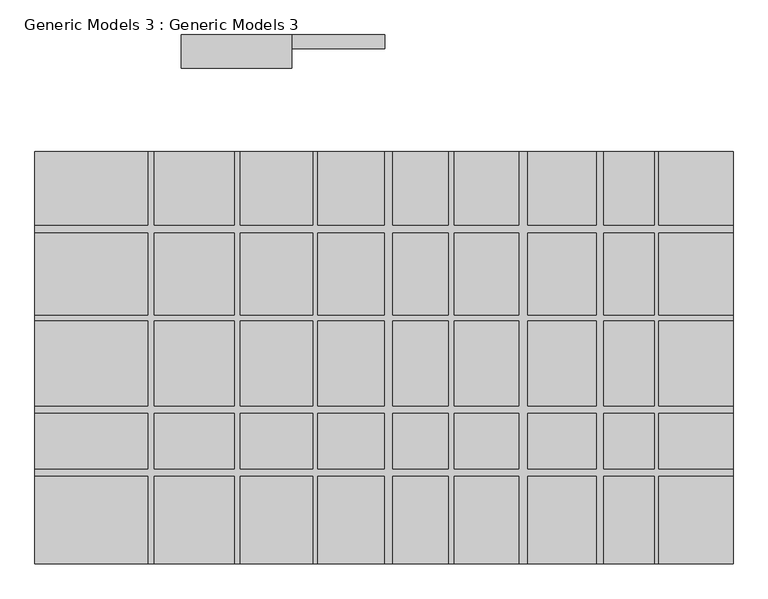
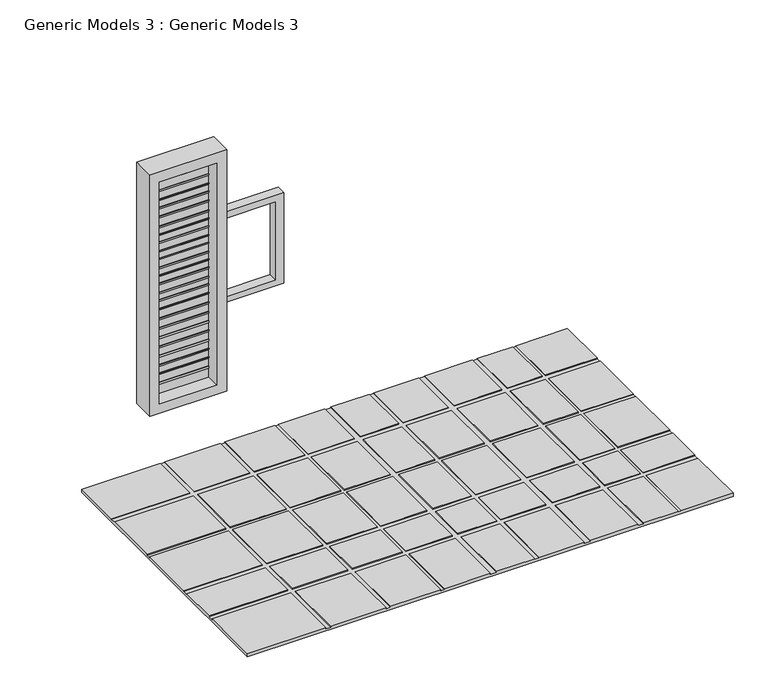
"""IFC4 building model written with IfcOpenShell, lengths in millimetres: proxy geometry, Generic Models 3 : Generic Models 3."""

from ifc_helpers import new_model, si_unit, frame, origin, place, context, project, spatial, polyline, outline, extrude, faceted_brep, source, transform, mapped, element, save


def generic_models_3_generic_models_3_2fa08359(model_context):
    return source(origin(), model_context, "Body", "SolidModel", [
        faceted_brep([(-20282.6509421, -24714.0121703, -199.9886332), (-20282.6509421, -24714.0121703, -304.8), (-4816.0838989, -24714.0121703, -304.8), (-4816.0838989, -24714.0121703, -199.9886332), (-6459.456614, -24714.0121703, -199.9886332), (-6459.456614, -24714.0121703, -225.3886332), (-6558.4876686, -24714.0121703, -225.3886332), (-6558.4876686, -24714.0121703, -199.9886332), (-7682.5837988, -24714.0121703, -199.9886332), (-7682.5837988, -24714.0121703, -225.3886332), (-7844.9819804, -24714.0121703, -225.3886332), (-7844.9819804, -24714.0121703, -199.9886332), (-9361.6851863, -24714.0121703, -199.9886332), (-9361.6851863, -24714.0121703, -225.3886332), (-9559.2287466, -24714.0121703, -225.3886332), (-9559.2287466, -24714.0121703, -199.9886332), (-10989.7031112, -24714.0121703, -199.9886332), (-10989.7031112, -24714.0121703, -225.3886332), (-11128.2513699, -24714.0121703, -225.3886332), (-11128.2513699, -24714.0121703, -199.9886332), (-12358.8798782, -24714.0121703, -199.9886332), (-12358.8798782, -24714.0121703, -225.3886332), (-12549.3674205, -24714.0121703, -225.3886332), (-12549.3674205, -24714.0121703, -199.9886332), (-14019.0040289, -24714.0121703, -199.9886332), (-14019.0040289, -24714.0121703, -225.3886332), (-14129.813477, -24714.0121703, -225.3886332), (-14129.813477, -24714.0121703, -199.9886332), (-15729.4103714, -24714.0121703, -199.9886332), (-15729.4103714, -24714.0121703, -225.3886332), (-15869.0039818, -24714.0121703, -225.3886332), (-15869.0039818, -24714.0121703, -199.9886332), (-17638.3624893, -24714.0121703, -199.9886332), (-17638.3624893, -24714.0121703, -225.3886332), (-17782.4676881, -24714.0121703, -225.3886332), (-17782.4676881, -24714.0121703, -199.9886332), (-4816.0838989, -15574.9202535, -199.9886332), (-4816.0838989, -15574.9202535, -304.8), (-20282.6509421, -15574.9202535, -304.8), (-20282.6509421, -15574.9202535, -199.9886332), (-17782.4676881, -15574.9202535, -199.9886332), (-17782.4676881, -15574.9202535, -225.3886332), (-17638.3624893, -15574.9202535, -225.3886332), (-17638.3624893, -15574.9202535, -199.9886332), (-15869.0039818, -15574.9202535, -199.9886332), (-15869.0039818, -15574.9202535, -225.3886332), (-15729.4103714, -15574.9202535, -225.3886332), (-15729.4103714, -15574.9202535, -199.9886332), (-14129.813477, -15574.9202535, -199.9886332), (-14129.813477, -15574.9202535, -225.3886332), (-14019.0040289, -15574.9202535, -225.3886332), (-14019.0040289, -15574.9202535, -199.9886332), (-12549.3674205, -15574.9202535, -199.9886332), (-12549.3674205, -15574.9202535, -225.3886332), (-12358.8798782, -15574.9202535, -225.3886332), (-12358.8798782, -15574.9202535, -199.9886332), (-11128.2513699, -15574.9202535, -199.9886332), (-11128.2513699, -15574.9202535, -225.3886332), (-10989.7031112, -15574.9202535, -225.3886332), (-10989.7031112, -15574.9202535, -199.9886332), (-9559.2287466, -15574.9202535, -199.9886332), (-9559.2287466, -15574.9202535, -225.3886332), (-9361.6851863, -15574.9202535, -225.3886332), (-9361.6851863, -15574.9202535, -199.9886332), (-7844.9819804, -15574.9202535, -199.9886332), (-7844.9819804, -15574.9202535, -225.3886332), (-7682.5837988, -15574.9202535, -225.3886332), (-7682.5837988, -15574.9202535, -199.9886332), (-6558.4876686, -15574.9202535, -199.9886332), (-6558.4876686, -15574.9202535, -225.3886332), (-6459.456614, -15574.9202535, -225.3886332), (-6459.456614, -15574.9202535, -199.9886332), (-20282.6509421, -22775.4634209, -199.9886332), (-20282.6509421, -22775.4634209, -225.3886332), (-20282.6509421, -22602.6183703, -225.3886332), (-20282.6509421, -22602.6183703, -199.9886332), (-20282.6509421, -21374.3729543, -199.9886332), (-20282.6509421, -21374.3729543, -225.3886332), (-20282.6509421, -21210.0078802, -225.3886332), (-20282.6509421, -21210.0078802, -199.9886332), (-20282.6509421, -19331.6285997, -199.9886332), (-20282.6509421, -19331.6285997, -225.3886332), (-20282.6509421, -19196.3153794, -225.3886332), (-20282.6509421, -19196.3153794, -199.9886332), (-20282.6509421, -17380.100746, -199.9886332), (-20282.6509421, -17380.100746, -225.3886332), (-20282.6509421, -17207.3737552, -225.3886332), (-20282.6509421, -17207.3737552, -199.9886332), (-4816.0838989, -17207.3737552, -199.9886332), (-4816.0838989, -17207.3737552, -225.3886332), (-4816.0838989, -17380.100746, -225.3886332), (-4816.0838989, -17380.100746, -199.9886332), (-4816.0838989, -19196.3153794, -199.9886332), (-4816.0838989, -19196.3153794, -225.3886332), (-4816.0838989, -19331.6285997, -225.3886332), (-4816.0838989, -19331.6285997, -199.9886332), (-4816.0838989, -21210.0078802, -199.9886332), (-4816.0838989, -21210.0078802, -225.3886332), (-4816.0838989, -21374.3729543, -225.3886332), (-4816.0838989, -21374.3729543, -199.9886332), (-4816.0838989, -22602.6183703, -199.9886332), (-4816.0838989, -22602.6183703, -225.3886332), (-4816.0838989, -22775.4634209, -225.3886332), (-4816.0838989, -22775.4634209, -199.9886332), (-6459.456614, -22775.4634209, -199.9886332), (-6558.4876686, -22775.4634209, -199.9886332), (-7682.5837988, -22775.4634209, -199.9886332), (-7844.9819804, -22775.4634209, -199.9886332), (-9361.6851863, -22775.4634209, -199.9886332), (-9559.2287466, -22775.4634209, -199.9886332), (-10989.7031112, -22775.4634209, -199.9886332), (-11128.2513699, -22775.4634209, -199.9886332), (-12358.8798782, -22775.4634209, -199.9886332), (-12549.3674205, -22775.4634209, -199.9886332), (-14019.0040289, -22775.4634209, -199.9886332), (-14129.813477, -22775.4634209, -199.9886332), (-15729.4103714, -22775.4634209, -199.9886332), (-15869.0039818, -22775.4634209, -199.9886332), (-17638.3624893, -22775.4634209, -199.9886332), (-17782.4676881, -22775.4634209, -199.9886332), (-17782.4676881, -17207.3737552, -199.9886332), (-17638.3624893, -17207.3737552, -199.9886332), (-15869.0039818, -17207.3737552, -199.9886332), (-15729.4103714, -17207.3737552, -199.9886332), (-14129.813477, -17207.3737552, -199.9886332), (-14019.0040289, -17207.3737552, -199.9886332), (-12549.3674205, -17207.3737552, -199.9886332), (-12358.8798782, -17207.3737552, -199.9886332), (-11128.2513699, -17207.3737552, -199.9886332), (-10989.7031112, -17207.3737552, -199.9886332), (-9559.2287466, -17207.3737552, -199.9886332), (-9361.6851863, -17207.3737552, -199.9886332), (-7844.9819804, -17207.3737552, -199.9886332), (-7682.5837988, -17207.3737552, -199.9886332), (-6558.4876686, -17207.3737552, -199.9886332), (-6459.456614, -17207.3737552, -199.9886332), (-17782.4676881, -22602.6183703, -199.9886332), (-17782.4676881, -21374.3729543, -199.9886332), (-17782.4676881, -21210.0078802, -199.9886332), (-17782.4676881, -19331.6285997, -199.9886332), (-17782.4676881, -19196.3153794, -199.9886332), (-17782.4676881, -17380.100746, -199.9886332), (-6459.456614, -17380.100746, -199.9886332), (-6459.456614, -19196.3153794, -199.9886332), (-6459.456614, -19331.6285997, -199.9886332), (-6459.456614, -21210.0078802, -199.9886332), (-6459.456614, -21374.3729543, -199.9886332), (-6459.456614, -22602.6183703, -199.9886332), (-15869.0039818, -19196.3153794, -199.9886332), (-15869.0039818, -17380.100746, -199.9886332), (-17638.3624893, -17380.100746, -199.9886332), (-17638.3624893, -19196.3153794, -199.9886332), (-15869.0039818, -21210.0078802, -199.9886332), (-15869.0039818, -19331.6285997, -199.9886332), (-17638.3624893, -19331.6285997, -199.9886332), (-17638.3624893, -21210.0078802, -199.9886332), (-15869.0039818, -22602.6183703, -199.9886332), (-15869.0039818, -21374.3729543, -199.9886332), (-17638.3624893, -21374.3729543, -199.9886332), (-17638.3624893, -22602.6183703, -199.9886332), (-14129.813477, -19196.3153794, -199.9886332), (-14129.813477, -17380.100746, -199.9886332), (-15729.4103714, -17380.100746, -199.9886332), (-15729.4103714, -19196.3153794, -199.9886332), (-14129.813477, -21210.0078802, -199.9886332), (-14129.813477, -19331.6285997, -199.9886332), (-15729.4103714, -19331.6285997, -199.9886332), (-15729.4103714, -21210.0078802, -199.9886332), (-14129.813477, -22602.6183703, -199.9886332), (-14129.813477, -21374.3729543, -199.9886332), (-15729.4103714, -21374.3729543, -199.9886332), (-15729.4103714, -22602.6183703, -199.9886332), (-12549.3674205, -19196.3153794, -199.9886332), (-12549.3674205, -17380.100746, -199.9886332), (-14019.0040289, -17380.100746, -199.9886332), (-14019.0040289, -19196.3153794, -199.9886332), (-12549.3674205, -21210.0078802, -199.9886332), (-12549.3674205, -19331.6285997, -199.9886332), (-14019.0040289, -19331.6285997, -199.9886332), (-14019.0040289, -21210.0078802, -199.9886332), (-12549.3674205, -22602.6183703, -199.9886332), (-12549.3674205, -21374.3729543, -199.9886332), (-14019.0040289, -21374.3729543, -199.9886332), (-14019.0040289, -22602.6183703, -199.9886332), (-11128.2513699, -19196.3153794, -199.9886332), (-11128.2513699, -17380.100746, -199.9886332), (-12358.8798782, -17380.100746, -199.9886332), (-12358.8798782, -19196.3153794, -199.9886332), (-11128.2513699, -21210.0078802, -199.9886332), (-11128.2513699, -19331.6285997, -199.9886332), (-12358.8798782, -19331.6285997, -199.9886332), (-12358.8798782, -21210.0078802, -199.9886332), (-11128.2513699, -22602.6183703, -199.9886332), (-11128.2513699, -21374.3729543, -199.9886332), (-12358.8798782, -21374.3729543, -199.9886332), (-12358.8798782, -22602.6183703, -199.9886332), (-9559.2287466, -19196.3153794, -199.9886332), (-9559.2287466, -17380.100746, -199.9886332), (-10989.7031112, -17380.100746, -199.9886332), (-10989.7031112, -19196.3153794, -199.9886332), (-9559.2287466, -21210.0078802, -199.9886332), (-9559.2287466, -19331.6285997, -199.9886332), (-10989.7031112, -19331.6285997, -199.9886332), (-10989.7031112, -21210.0078802, -199.9886332), (-9559.2287466, -22602.6183703, -199.9886332), (-9559.2287466, -21374.3729543, -199.9886332), (-10989.7031112, -21374.3729543, -199.9886332), (-10989.7031112, -22602.6183703, -199.9886332), (-7844.9819804, -19196.3153794, -199.9886332), (-7844.9819804, -17380.100746, -199.9886332), (-9361.6851863, -17380.100746, -199.9886332), (-9361.6851863, -19196.3153794, -199.9886332), (-7844.9819804, -21210.0078802, -199.9886332), (-7844.9819804, -19331.6285997, -199.9886332), (-9361.6851863, -19331.6285997, -199.9886332), (-9361.6851863, -21210.0078802, -199.9886332), (-7844.9819804, -22602.6183703, -199.9886332), (-7844.9819804, -21374.3729543, -199.9886332), (-9361.6851863, -21374.3729543, -199.9886332), (-9361.6851863, -22602.6183703, -199.9886332), (-6558.4876686, -19196.3153794, -199.9886332), (-6558.4876686, -17380.100746, -199.9886332), (-7682.5837988, -17380.100746, -199.9886332), (-7682.5837988, -19196.3153794, -199.9886332), (-6558.4876686, -21210.0078802, -199.9886332), (-6558.4876686, -19331.6285997, -199.9886332), (-7682.5837988, -19331.6285997, -199.9886332), (-7682.5837988, -21210.0078802, -199.9886332), (-6558.4876686, -22602.6183703, -199.9886332), (-6558.4876686, -21374.3729543, -199.9886332), (-7682.5837988, -21374.3729543, -199.9886332), (-7682.5837988, -22602.6183703, -199.9886332), (-17638.3624893, -22775.4634209, -225.3886332), (-15869.0039818, -22775.4634209, -225.3886332), (-15729.4103714, -22775.4634209, -225.3886332), (-14129.813477, -22775.4634209, -225.3886332), (-14019.0040289, -22775.4634209, -225.3886332), (-12549.3674205, -22775.4634209, -225.3886332), (-12358.8798782, -22775.4634209, -225.3886332), (-11128.2513699, -22775.4634209, -225.3886332), (-10989.7031112, -22775.4634209, -225.3886332), (-9559.2287466, -22775.4634209, -225.3886332), (-9361.6851863, -22775.4634209, -225.3886332), (-7844.9819804, -22775.4634209, -225.3886332), (-7682.5837988, -22775.4634209, -225.3886332), (-6558.4876686, -22775.4634209, -225.3886332), (-6459.456614, -22775.4634209, -225.3886332), (-6459.456614, -22602.6183703, -225.3886332), (-6459.456614, -21374.3729543, -225.3886332), (-6459.456614, -21210.0078802, -225.3886332), (-6459.456614, -19331.6285997, -225.3886332), (-6459.456614, -19196.3153794, -225.3886332), (-6459.456614, -17380.100746, -225.3886332), (-6459.456614, -17207.3737552, -225.3886332), (-6558.4876686, -17207.3737552, -225.3886332), (-7682.5837988, -17207.3737552, -225.3886332), (-7844.9819804, -17207.3737552, -225.3886332), (-9361.6851863, -17207.3737552, -225.3886332), (-9559.2287466, -17207.3737552, -225.3886332), (-10989.7031112, -17207.3737552, -225.3886332), (-11128.2513699, -17207.3737552, -225.3886332), (-12358.8798782, -17207.3737552, -225.3886332), (-12549.3674205, -17207.3737552, -225.3886332), (-14019.0040289, -17207.3737552, -225.3886332), (-14129.813477, -17207.3737552, -225.3886332), (-15729.4103714, -17207.3737552, -225.3886332), (-15869.0039818, -17207.3737552, -225.3886332), (-17638.3624893, -17207.3737552, -225.3886332), (-17782.4676881, -17207.3737552, -225.3886332), (-17782.4676881, -17380.100746, -225.3886332), (-17782.4676881, -19196.3153794, -225.3886332), (-17782.4676881, -19331.6285997, -225.3886332), (-17782.4676881, -21210.0078802, -225.3886332), (-17782.4676881, -21374.3729543, -225.3886332), (-17782.4676881, -22602.6183703, -225.3886332), (-17782.4676881, -22775.4634209, -225.3886332), (-17638.3624893, -19196.3153794, -225.3886332), (-17638.3624893, -17380.100746, -225.3886332), (-15869.0039818, -17380.100746, -225.3886332), (-15869.0039818, -19196.3153794, -225.3886332), (-17638.3624893, -21210.0078802, -225.3886332), (-17638.3624893, -19331.6285997, -225.3886332), (-15869.0039818, -19331.6285997, -225.3886332), (-15869.0039818, -21210.0078802, -225.3886332), (-17638.3624893, -22602.6183703, -225.3886332), (-17638.3624893, -21374.3729543, -225.3886332), (-15869.0039818, -21374.3729543, -225.3886332), (-15869.0039818, -22602.6183703, -225.3886332), (-15729.4103714, -19196.3153794, -225.3886332), (-15729.4103714, -17380.100746, -225.3886332), (-14129.813477, -17380.100746, -225.3886332), (-14129.813477, -19196.3153794, -225.3886332), (-15729.4103714, -21210.0078802, -225.3886332), (-15729.4103714, -19331.6285997, -225.3886332), (-14129.813477, -19331.6285997, -225.3886332), (-14129.813477, -21210.0078802, -225.3886332), (-15729.4103714, -22602.6183703, -225.3886332), (-15729.4103714, -21374.3729543, -225.3886332), (-14129.813477, -21374.3729543, -225.3886332), (-14129.813477, -22602.6183703, -225.3886332), (-14019.0040289, -19196.3153794, -225.3886332), (-14019.0040289, -17380.100746, -225.3886332), (-12549.3674205, -17380.100746, -225.3886332), (-12549.3674205, -19196.3153794, -225.3886332), (-14019.0040289, -21210.0078802, -225.3886332), (-14019.0040289, -19331.6285997, -225.3886332), (-12549.3674205, -19331.6285997, -225.3886332), (-12549.3674205, -21210.0078802, -225.3886332), (-14019.0040289, -22602.6183703, -225.3886332), (-14019.0040289, -21374.3729543, -225.3886332), (-12549.3674205, -21374.3729543, -225.3886332), (-12549.3674205, -22602.6183703, -225.3886332), (-12358.8798782, -19196.3153794, -225.3886332), (-12358.8798782, -17380.100746, -225.3886332), (-11128.2513699, -17380.100746, -225.3886332), (-11128.2513699, -19196.3153794, -225.3886332), (-12358.8798782, -21210.0078802, -225.3886332), (-12358.8798782, -19331.6285997, -225.3886332), (-11128.2513699, -19331.6285997, -225.3886332), (-11128.2513699, -21210.0078802, -225.3886332), (-12358.8798782, -22602.6183703, -225.3886332), (-12358.8798782, -21374.3729543, -225.3886332), (-11128.2513699, -21374.3729543, -225.3886332), (-11128.2513699, -22602.6183703, -225.3886332), (-10989.7031112, -19196.3153794, -225.3886332), (-10989.7031112, -17380.100746, -225.3886332), (-9559.2287466, -17380.100746, -225.3886332), (-9559.2287466, -19196.3153794, -225.3886332), (-10989.7031112, -21210.0078802, -225.3886332), (-10989.7031112, -19331.6285997, -225.3886332), (-9559.2287466, -19331.6285997, -225.3886332), (-9559.2287466, -21210.0078802, -225.3886332), (-10989.7031112, -22602.6183703, -225.3886332), (-10989.7031112, -21374.3729543, -225.3886332), (-9559.2287466, -21374.3729543, -225.3886332), (-9559.2287466, -22602.6183703, -225.3886332), (-9361.6851863, -19196.3153794, -225.3886332), (-9361.6851863, -17380.100746, -225.3886332), (-7844.9819804, -17380.100746, -225.3886332), (-7844.9819804, -19196.3153794, -225.3886332), (-9361.6851863, -21210.0078802, -225.3886332), (-9361.6851863, -19331.6285997, -225.3886332), (-7844.9819804, -19331.6285997, -225.3886332), (-7844.9819804, -21210.0078802, -225.3886332), (-9361.6851863, -22602.6183703, -225.3886332), (-9361.6851863, -21374.3729543, -225.3886332), (-7844.9819804, -21374.3729543, -225.3886332), (-7844.9819804, -22602.6183703, -225.3886332), (-7682.5837988, -19196.3153794, -225.3886332), (-7682.5837988, -17380.100746, -225.3886332), (-6558.4876686, -17380.100746, -225.3886332), (-6558.4876686, -19196.3153794, -225.3886332), (-7682.5837988, -21210.0078802, -225.3886332), (-7682.5837988, -19331.6285997, -225.3886332), (-6558.4876686, -19331.6285997, -225.3886332), (-6558.4876686, -21210.0078802, -225.3886332), (-7682.5837988, -22602.6183703, -225.3886332), (-7682.5837988, -21374.3729543, -225.3886332), (-6558.4876686, -21374.3729543, -225.3886332), (-6558.4876686, -22602.6183703, -225.3886332)], [[[0, 1, 2, 3, 4, 5, 6, 7, 8, 9, 10, 11, 12, 13, 14, 15, 16, 17, 18, 19, 20, 21, 22, 23, 24, 25, 26, 27, 28, 29, 30, 31, 32, 33, 34, 35]], [[36, 37, 38, 39, 40, 41, 42, 43, 44, 45, 46, 47, 48, 49, 50, 51, 52, 53, 54, 55, 56, 57, 58, 59, 60, 61, 62, 63, 64, 65, 66, 67, 68, 69, 70, 71]], [[1, 0, 72, 73, 74, 75, 76, 77, 78, 79, 80, 81, 82, 83, 84, 85, 86, 87, 39, 38]], [[2, 1, 38, 37]], [[3, 2, 37, 36, 88, 89, 90, 91, 92, 93, 94, 95, 96, 97, 98, 99, 100, 101, 102, 103]], [[4, 3, 103, 104]], [[8, 7, 105, 106]], [[12, 11, 107, 108]], [[16, 15, 109, 110]], [[20, 19, 111, 112]], [[24, 23, 113, 114]], [[28, 27, 115, 116]], [[32, 31, 117, 118]], [[0, 35, 119, 72]], [[40, 39, 87, 120]], [[44, 43, 121, 122]], [[48, 47, 123, 124]], [[52, 51, 125, 126]], [[56, 55, 127, 128]], [[60, 59, 129, 130]], [[64, 63, 131, 132]], [[68, 67, 133, 134]], [[36, 71, 135, 88]], [[76, 75, 136, 137]], [[80, 79, 138, 139]], [[84, 83, 140, 141]], [[92, 91, 142, 143]], [[96, 95, 144, 145]], [[100, 99, 146, 147]], [[148, 149, 150, 151]], [[152, 153, 154, 155]], [[156, 157, 158, 159]], [[160, 161, 162, 163]], [[164, 165, 166, 167]], [[168, 169, 170, 171]], [[172, 173, 174, 175]], [[176, 177, 178, 179]], [[180, 181, 182, 183]], [[184, 185, 186, 187]], [[188, 189, 190, 191]], [[192, 193, 194, 195]], [[196, 197, 198, 199]], [[200, 201, 202, 203]], [[204, 205, 206, 207]], [[208, 209, 210, 211]], [[212, 213, 214, 215]], [[216, 217, 218, 219]], [[220, 221, 222, 223]], [[224, 225, 226, 227]], [[228, 229, 230, 231]], [[34, 33, 232, 233, 30, 29, 234, 235, 26, 25, 236, 237, 22, 21, 238, 239, 18, 17, 240, 241, 14, 13, 242, 243, 10, 9, 244, 245, 6, 5, 246, 102, 101, 247, 248, 98, 97, 249, 250, 94, 93, 251, 252, 90, 89, 253, 70, 69, 254, 255, 66, 65, 256, 257, 62, 61, 258, 259, 58, 57, 260, 261, 54, 53, 262, 263, 50, 49, 264, 265, 46, 45, 266, 267, 42, 41, 268, 86, 85, 269, 270, 82, 81, 271, 272, 78, 77, 273, 274, 74, 73, 275], [276, 277, 278, 279], [280, 281, 282, 283], [284, 285, 286, 287], [288, 289, 290, 291], [292, 293, 294, 295], [296, 297, 298, 299], [300, 301, 302, 303], [304, 305, 306, 307], [308, 309, 310, 311], [312, 313, 314, 315], [316, 317, 318, 319], [320, 321, 322, 323], [324, 325, 326, 327], [328, 329, 330, 331], [332, 333, 334, 335], [336, 337, 338, 339], [340, 341, 342, 343], [344, 345, 346, 347], [348, 349, 350, 351], [352, 353, 354, 355], [356, 357, 358, 359]], [[33, 32, 118, 232]], [[43, 42, 267, 121]], [[151, 150, 277, 276]], [[155, 154, 281, 280]], [[159, 158, 285, 284]], [[35, 34, 275, 119]], [[41, 40, 120, 268]], [[141, 140, 270, 269]], [[139, 138, 272, 271]], [[137, 136, 274, 273]], [[29, 28, 116, 234]], [[47, 46, 265, 123]], [[163, 162, 289, 288]], [[167, 166, 293, 292]], [[171, 170, 297, 296]], [[31, 30, 233, 117]], [[45, 44, 122, 266]], [[149, 148, 279, 278]], [[153, 152, 283, 282]], [[157, 156, 287, 286]], [[25, 24, 114, 236]], [[51, 50, 263, 125]], [[175, 174, 301, 300]], [[179, 178, 305, 304]], [[183, 182, 309, 308]], [[27, 26, 235, 115]], [[49, 48, 124, 264]], [[161, 160, 291, 290]], [[165, 164, 295, 294]], [[169, 168, 299, 298]], [[21, 20, 112, 238]], [[55, 54, 261, 127]], [[187, 186, 313, 312]], [[191, 190, 317, 316]], [[195, 194, 321, 320]], [[23, 22, 237, 113]], [[53, 52, 126, 262]], [[173, 172, 303, 302]], [[177, 176, 307, 306]], [[181, 180, 311, 310]], [[17, 16, 110, 240]], [[59, 58, 259, 129]], [[199, 198, 325, 324]], [[203, 202, 329, 328]], [[207, 206, 333, 332]], [[19, 18, 239, 111]], [[57, 56, 128, 260]], [[185, 184, 315, 314]], [[189, 188, 319, 318]], [[193, 192, 323, 322]], [[13, 12, 108, 242]], [[63, 62, 257, 131]], [[211, 210, 337, 336]], [[215, 214, 341, 340]], [[219, 218, 345, 344]], [[15, 14, 241, 109]], [[61, 60, 130, 258]], [[197, 196, 327, 326]], [[201, 200, 331, 330]], [[205, 204, 335, 334]], [[9, 8, 106, 244]], [[67, 66, 255, 133]], [[223, 222, 349, 348]], [[227, 226, 353, 352]], [[231, 230, 357, 356]], [[11, 10, 243, 107]], [[65, 64, 132, 256]], [[209, 208, 339, 338]], [[213, 212, 343, 342]], [[217, 216, 347, 346]], [[5, 4, 104, 246]], [[71, 70, 253, 135]], [[143, 142, 252, 251]], [[145, 144, 250, 249]], [[147, 146, 248, 247]], [[7, 6, 245, 105]], [[69, 68, 134, 254]], [[221, 220, 351, 350]], [[225, 224, 355, 354]], [[229, 228, 359, 358]], [[90, 252, 142, 91]], [[269, 85, 84, 141]], [[278, 277, 150, 149]], [[290, 289, 162, 161]], [[302, 301, 174, 173]], [[314, 313, 186, 185]], [[326, 325, 198, 197]], [[338, 337, 210, 209]], [[350, 349, 222, 221]], [[253, 89, 88, 135]], [[255, 254, 134, 133]], [[257, 256, 132, 131]], [[259, 258, 130, 129]], [[261, 260, 128, 127]], [[263, 262, 126, 125]], [[265, 264, 124, 123]], [[267, 266, 122, 121]], [[86, 268, 120, 87]], [[94, 250, 144, 95]], [[271, 81, 80, 139]], [[282, 281, 154, 153]], [[294, 293, 166, 165]], [[306, 305, 178, 177]], [[318, 317, 190, 189]], [[330, 329, 202, 201]], [[342, 341, 214, 213]], [[354, 353, 226, 225]], [[251, 93, 92, 143]], [[82, 270, 140, 83]], [[276, 279, 148, 151]], [[288, 291, 160, 163]], [[300, 303, 172, 175]], [[312, 315, 184, 187]], [[324, 327, 196, 199]], [[336, 339, 208, 211]], [[348, 351, 220, 223]], [[98, 248, 146, 99]], [[273, 77, 76, 137]], [[286, 285, 158, 157]], [[298, 297, 170, 169]], [[310, 309, 182, 181]], [[322, 321, 194, 193]], [[334, 333, 206, 205]], [[346, 345, 218, 217]], [[358, 357, 230, 229]], [[249, 97, 96, 145]], [[78, 272, 138, 79]], [[280, 283, 152, 155]], [[292, 295, 164, 167]], [[304, 307, 176, 179]], [[316, 319, 188, 191]], [[328, 331, 200, 203]], [[340, 343, 212, 215]], [[352, 355, 224, 227]], [[233, 232, 118, 117]], [[235, 234, 116, 115]], [[237, 236, 114, 113]], [[239, 238, 112, 111]], [[241, 240, 110, 109]], [[243, 242, 108, 107]], [[245, 244, 106, 105]], [[102, 246, 104, 103]], [[275, 73, 72, 119]], [[247, 101, 100, 147]], [[74, 274, 136, 75]], [[284, 287, 156, 159]], [[296, 299, 168, 171]], [[308, 311, 180, 183]], [[320, 323, 192, 195]], [[332, 335, 204, 207]], [[344, 347, 216, 219]], [[356, 359, 228, 231]]]),
        extrude(outline(polyline([(-14922.5310076, -13317.4040375), (-16751.3310076, -13317.4040375), (-16751.3310076, -13292.0040375), (-14922.5310076, -13292.0040375), (-14922.5310076, -13317.4040375)])), frame((0.0, 0.0, 7140.453118), z_axis=(0.0, 0.0, 1.0), x_axis=(1.0, 0.0, 0.0)), (0.0, 0.0, 1.0), 47.2445904),
        extrude(outline(polyline([(-14922.5310076, -13317.4040375), (-16751.3310076, -13317.4040375), (-16751.3310076, -13292.0040375), (-14922.5310076, -13292.0040375), (-14922.5310076, -13317.4040375)])), frame((0.0, 0.0, 6836.9032708), z_axis=(0.0, 0.0, 1.0), x_axis=(1.0, 0.0, 0.0)), (0.0, 0.0, 1.0), 44.4473087),
        extrude(outline(polyline([(-14922.5310076, -13317.4040375), (-16751.3310076, -13317.4040375), (-16751.3310076, -13292.0040375), (-14922.5310076, -13292.0040375), (-14922.5310076, -13317.4040375)])), frame((0.0, 0.0, 6553.1243), z_axis=(0.0, 0.0, 1.0), x_axis=(1.0, 0.0, 0.0)), (0.0, 0.0, 1.0), 54.7043799),
        extrude(outline(polyline([(-14922.5310076, -13317.4040375), (-16751.3310076, -13317.4040375), (-16751.3310076, -13292.0040375), (-14922.5310076, -13292.0040375), (-14922.5310076, -13317.4040375)])), frame((0.0, 0.0, 6252.2502106), z_axis=(0.0, 0.0, 1.0), x_axis=(1.0, 0.0, 0.0)), (0.0, 0.0, 1.0), 54.7043799),
        extrude(outline(polyline([(-14922.5310076, -13317.4040375), (-16751.3310076, -13317.4040375), (-16751.3310076, -13292.0040375), (-14922.5310076, -13292.0040375), (-14922.5310076, -13317.4040375)])), frame((0.0, 0.0, 5920.6049074), z_axis=(0.0, 0.0, 1.0), x_axis=(1.0, 0.0, 0.0)), (0.0, 0.0, 1.0), 51.2853562),
        extrude(outline(polyline([(-14922.5310076, -13317.4040375), (-16751.3310076, -13317.4040375), (-16751.3310076, -13292.0040375), (-14922.5310076, -13292.0040375), (-14922.5310076, -13317.4040375)])), frame((0.0, 0.0, 5665.1799199), z_axis=(0.0, 0.0, 1.0), x_axis=(1.0, 0.0, 0.0)), (0.0, 0.0, 1.0), 33.5754545),
        extrude(outline(polyline([(-14922.5310076, -13317.4040375), (-16751.3310076, -13317.4040375), (-16751.3310076, -13292.0040375), (-14922.5310076, -13292.0040375), (-14922.5310076, -13317.4040375)])), frame((0.0, 0.0, 5398.9822727), z_axis=(0.0, 0.0, 1.0), x_axis=(1.0, 0.0, 0.0)), (0.0, 0.0, 1.0), 38.842263),
        extrude(outline(polyline([(-14922.5310076, -13317.4040375), (-16751.3310076, -13317.4040375), (-16751.3310076, -13292.0040375), (-14922.5310076, -13292.0040375), (-14922.5310076, -13317.4040375)])), frame((0.0, 0.0, 5102.019423), z_axis=(0.0, 0.0, 1.0), x_axis=(1.0, 0.0, 0.0)), (0.0, 0.0, 1.0), 38.6498336),
        extrude(outline(polyline([(-14922.5310076, -13317.4040375), (-16751.3310076, -13317.4040375), (-16751.3310076, -13292.0040375), (-14922.5310076, -13292.0040375), (-14922.5310076, -13317.4040375)])), frame((0.0, 0.0, 4848.1196978), z_axis=(0.0, 0.0, 1.0), x_axis=(1.0, 0.0, 0.0)), (0.0, 0.0, 1.0), 33.8929799),
        extrude(outline(polyline([(-14922.5310076, -13317.4040375), (-16751.3310076, -13317.4040375), (-16751.3310076, -13292.0040375), (-14922.5310076, -13292.0040375), (-14922.5310076, -13317.4040375)])), frame((0.0, 0.0, 4539.6895855), z_axis=(0.0, 0.0, 1.0), x_axis=(1.0, 0.0, 0.0)), (0.0, 0.0, 1.0), 45.1534114),
        extrude(outline(polyline([(-14922.5310076, -13317.4040375), (-16751.3310076, -13317.4040375), (-16751.3310076, -13292.0040375), (-14922.5310076, -13292.0040375), (-14922.5310076, -13317.4040375)])), frame((0.0, 0.0, 4282.8595583), z_axis=(0.0, 0.0, 1.0), x_axis=(1.0, 0.0, 0.0)), (0.0, 0.0, 1.0), 39.7963461),
        extrude(outline(polyline([(-14922.5310076, -13317.4040375), (-16751.3310076, -13317.4040375), (-16751.3310076, -13292.0040375), (-14922.5310076, -13292.0040375), (-14922.5310076, -13317.4040375)])), frame((0.0, 0.0, 3995.7999113), z_axis=(0.0, 0.0, 1.0), x_axis=(1.0, 0.0, 0.0)), (0.0, 0.0, 1.0), 57.5140898),
        extrude(outline(polyline([(-14922.5310076, -13317.4040375), (-16751.3310076, -13317.4040375), (-16751.3310076, -13292.0040375), (-14922.5310076, -13292.0040375), (-14922.5310076, -13317.4040375)])), frame((0.0, 0.0, 3693.9524739), z_axis=(0.0, 0.0, 1.0), x_axis=(1.0, 0.0, 0.0)), (0.0, 0.0, 1.0), 44.3929462),
        extrude(outline(polyline([(-14922.5310076, -13317.4040375), (-16751.3310076, -13317.4040375), (-16751.3310076, -13292.0040375), (-14922.5310076, -13292.0040375), (-14922.5310076, -13317.4040375)])), frame((0.0, 0.0, 3437.5256931), z_axis=(0.0, 0.0, 1.0), x_axis=(1.0, 0.0, 0.0)), (0.0, 0.0, 1.0), 52.3981513),
        extrude(outline(polyline([(-14922.5310076, -13317.4040375), (-16751.3310076, -13317.4040375), (-16751.3310076, -13292.0040375), (-14922.5310076, -13292.0040375), (-14922.5310076, -13317.4040375)])), frame((0.0, 0.0, 3153.7467224), z_axis=(0.0, 0.0, 1.0), x_axis=(1.0, 0.0, 0.0)), (0.0, 0.0, 1.0), 41.0282849),
        extrude(outline(polyline([(-14922.5310076, -13317.4040375), (-16751.3310076, -13317.4040375), (-16751.3310076, -13292.0040375), (-14922.5310076, -13292.0040375), (-14922.5310076, -13317.4040375)])), frame((0.0, 0.0, 2822.1014192), z_axis=(0.0, 0.0, 1.0), x_axis=(1.0, 0.0, 0.0)), (0.0, 0.0, 1.0), 51.2853562),
        extrude(outline(polyline([(-14922.5310076, -13317.4040375), (-16751.3310076, -13317.4040375), (-16751.3310076, -13292.0040375), (-14922.5310076, -13292.0040375), (-14922.5310076, -13317.4040375)])), frame((0.0, 0.0, 2491.9743896), z_axis=(0.0, 0.0, 1.0), x_axis=(1.0, 0.0, 0.0)), (0.0, 0.0, 1.0), 56.6051301),
        extrude(outline(polyline([(-14922.5310076, -13317.4040375), (-16751.3310076, -13317.4040375), (-16751.3310076, -13292.0040375), (-14922.5310076, -13292.0040375), (-14922.5310076, -13317.4040375)])), frame((0.0, 0.0, 2179.3249553), z_axis=(0.0, 0.0, 1.0), x_axis=(1.0, 0.0, 0.0)), (0.0, 0.0, 1.0), 61.5424274),
        extrude(outline(polyline([(-14922.5310076, -13317.4040375), (-16751.3310076, -13317.4040375), (-16751.3310076, -13292.0040375), (-14922.5310076, -13292.0040375), (-14922.5310076, -13317.4040375)])), frame((0.0, 0.0, 1875.0318421), z_axis=(0.0, 0.0, 1.0), x_axis=(1.0, 0.0, 0.0)), (0.0, 0.0, 1.0), 51.2853562),
        extrude(outline(polyline([(-14922.5310076, -13317.4040375), (-16751.3310076, -13317.4040375), (-16751.3310076, -13292.0040375), (-14922.5310076, -13292.0040375), (-14922.5310076, -13317.4040375)])), frame((0.0, 0.0, 1560.4816577), z_axis=(0.0, 0.0, 1.0), x_axis=(1.0, 0.0, 0.0)), (0.0, 0.0, 1.0), 54.7043799),
        extrude(outline(polyline([(-14922.5310076, -13317.4040375), (-16751.3310076, -13317.4040375), (-16751.3310076, -13292.0040375), (-14922.5310076, -13292.0040375), (-14922.5310076, -13317.4040375)])), frame((0.0, 0.0, 1259.6075682), z_axis=(0.0, 0.0, 1.0), x_axis=(1.0, 0.0, 0.0)), (0.0, 0.0, 1.0), 47.8663324),
        extrude(outline(polyline([(-14922.5310076, -13317.4040375), (-16751.3310076, -13317.4040375), (-16751.3310076, -13292.0040375), (-14922.5310076, -13292.0040375), (-14922.5310076, -13317.4040375)])), frame((0.0, 0.0, 980.0431547), z_axis=(0.0, 0.0, 1.0), x_axis=(1.0, 0.0, 0.0)), (0.0, 0.0, 1.0), 39.9495254),
        extrude(outline(polyline([(-14922.5310076, -13317.4040375), (-16751.3310076, -13317.4040375), (-16751.3310076, -13292.0040375), (-14922.5310076, -13292.0040375), (-14922.5310076, -13317.4040375)])), frame((0.0, 0.0, 653.2824441), z_axis=(0.0, 0.0, 1.0), x_axis=(1.0, 0.0, 0.0)), (0.0, 0.0, 1.0), 54.7218305),
        extrude(outline(polyline([(5698.7553745, -12530.5912799), (5698.7553745, -14590.3624893), (5485.7911654, -14590.3624893), (5485.7911654, -12786.9624893), (2844.1911654, -12786.9624893), (2844.1911654, -14590.3624893), (2655.984893, -14590.3624893), (2655.984893, -12530.5912799), (5698.7553745, -12530.5912799)])), frame((0.0, -13292.0040375, 0.0), z_axis=(0.0, 1.0, 0.0), x_axis=(0.0, 0.0, 1.0)), (0.0, 0.0, 1.0), 304.8),
        faceted_brep([(-17045.3354046, -13723.8040375, 8130.7786353), (-17045.3354046, -13723.8040375, 0.0), (-14590.3624893, -13723.8040375, 0.0), (-14590.3624893, -13723.8040375, 8130.7786353), (-14922.5310076, -13723.8040375, 7787.1140011), (-14922.5310076, -13723.8040375, 319.5140011), (-16751.3310076, -13723.8040375, 319.5140011), (-16751.3310076, -13723.8040375, 7787.1140011), (-17045.3354046, -12987.2040375, 8130.7786353), (-14590.3624893, -12987.2040375, 8130.7786353), (-14590.3624893, -12987.2040375, 0.0), (-17045.3354046, -12987.2040375, 0.0), (-14922.5310076, -13292.0040375, 7787.1140011), (-16751.3310076, -13292.0040375, 7787.1140011), (-16751.3310076, -13292.0040375, 7510.2281293), (-14922.5310076, -13292.0040375, 7510.2281293), (-16751.3310076, -13292.0040375, 319.5140011), (-14922.5310076, -13292.0040375, 319.5140011), (-14922.5310076, -13292.0040375, 7453.5501179), (-16751.3310076, -13292.0040375, 7453.5501179), (-14922.5310076, -13266.6040375, 7510.2281293), (-14922.5310076, -13266.6040375, 7453.5501179), (-16751.3310076, -13266.6040375, 7453.5501179), (-16751.3310076, -13266.6040375, 7510.2281293)], [[[0, 1, 2, 3], [4, 5, 6, 7]], [[8, 9, 10, 11]], [[1, 0, 8, 11]], [[2, 1, 11, 10]], [[3, 2, 10, 9]], [[0, 3, 9, 8]], [[12, 13, 14, 15]], [[16, 17, 18, 19]], [[17, 5, 4, 12, 15, 20, 21, 18]], [[17, 16, 6, 5]], [[6, 16, 19, 22, 23, 14, 13, 7]], [[13, 12, 4, 7]], [[20, 23, 22, 21]], [[21, 22, 19, 18]], [[23, 20, 15, 14]]]),
    ])


if __name__ == "__main__":
    model = new_model("IFC4")
    model_context = context("Model", 3, world=origin())
    ifc_project = project(units=[si_unit("LENGTHUNIT", "METRE", prefix="MILLI")], contexts=[model_context])
    site = spatial("IfcSite", under=ifc_project)
    building = spatial("IfcBuilding", under=site)
    placement = place(None, origin())
    generic_models_3_generic_models_3_shape = generic_models_3_generic_models_3_2fa08359(model_context)
    element("IfcBuildingElementProxy", 1, Name="Generic Models 3 : Generic Models 3", ObjectType="Generic Models 3 : Generic Models 3", at=placement, inside=building, context=model_context, shape_type="MappedRepresentation", body=[
        mapped(generic_models_3_generic_models_3_shape, transform((0.0, 0.0, 0.0), x_axis=(1.0, 0.0, 0.0), y_axis=(0.0, 1.0, 0.0), z_axis=(0.0, 0.0, 1.0))),
    ])
    save(model, "model.ifc")
